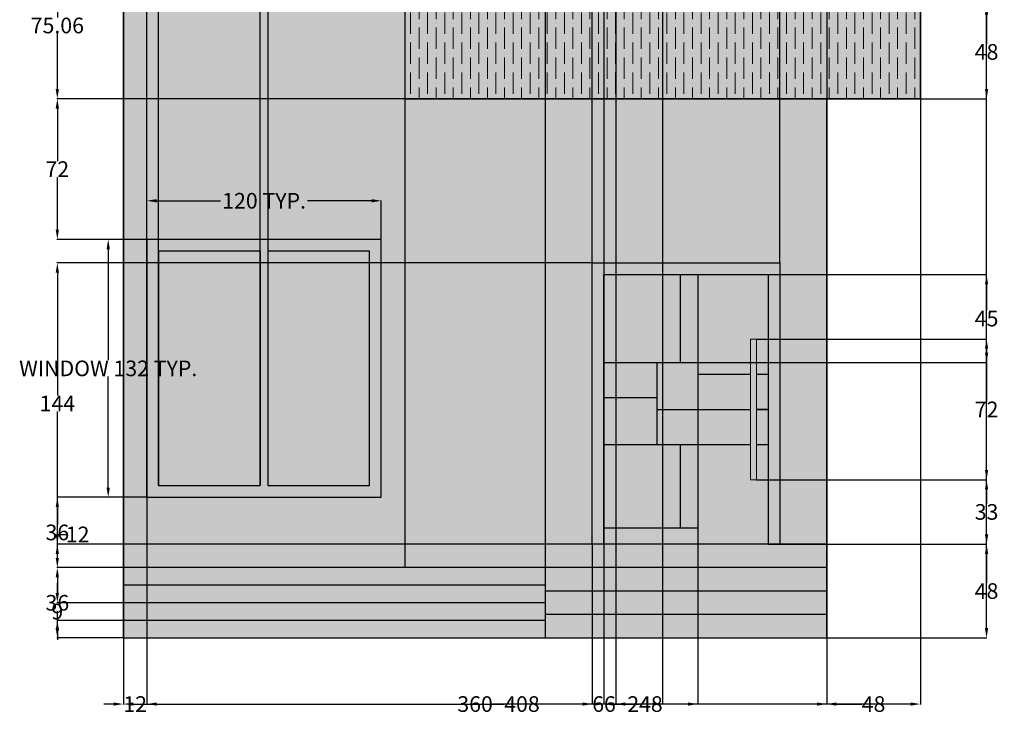
# Model space of a CAD drawing. Units: inches. Extents: x 137 to 641, y 88 to 838.
# Tile 1 of 2: x 137 to 641, y 88 to 444. Entities that reach past the tile are written whole.
import ezdxf

# ---------------------------------------------------------------- set-up
doc = ezdxf.new("R2010")
doc.units = ezdxf.units.IN
doc.header["$MEASUREMENT"] = 0
doc.layers.get('0').update_dxf_attribs({"color": 250})
for name, color, linetype, lineweight in [('A-ANNO-DIMS', 2, 'Continuous', 18), ('A-DOOR', 250, 'Continuous', 25), ('A-DOOR-HRDW', 250, 'Continuous', 18), ('A-ELEV-TRIM-PATT', 18, 'Continuous', 13), ('A-FLOR-BALC', 250, 'Continuous', 35), ('A-FLOR-BALC-PATT', 250, 'Continuous', 13), ('A-FLOR-STRS', 250, 'Continuous', 25), ('A-GLAZ', 250, 'Continuous', 25), ('A-GLAZ-PATT', 250, 'Continuous', 13), ('A-WALL', 250, 'Continuous', 35), ('A-WALL-CLAD', 250, 'Continuous', 25), ('A-WALL-PLIN', 251, 'Continuous', 25)]:
    doc.layers.add(name, color=color, linetype=linetype, lineweight=lineweight)
for name, color, linetype, lineweight, true_color in [('A-DOOR-PATT', 251, 'Continuous', 13, 0x636466), ('A-FLOR-BALC-FILL', 89, 'Continuous', 13, 0x333e19), ('A-FLOR-STRS-PATT', 9, 'Continuous', 13, 0xe0c8a3), ('A-WALL-CLAD-FILL', 51, 'Continuous', 13, 0xfff4a4), ('A-WALL-CLAD-PATT', 21, 'Continuous', 13, 0xe2a688), ('A-WALL-PATT', 254, 'Continuous', 13, 0xd7ebd2), ('A-WALL-PLIN-PATT', 108, 'Continuous', 13, 0x0a0f0b)]:
    doc.layers.add(name, color=color, linetype=linetype, lineweight=lineweight, true_color=true_color)
doc.styles.get("Standard").update_dxf_attribs({"font": 'arial.ttf'})
doc.dimstyles.get("Standard").update_dxf_attribs({"dimtxt": 8, "dimasz": 5, "dimexe": 0.18, "dimexo": 0.0625, "dimgap": 0.09, "dimtad": 0, "dimtih": 1, "dimtoh": 1, "dimdec": 0, "dimzin": 0, "dimdsep": 46, "dimlunit": 3, "dimtxsty": 'Standard', "dimcen": 0.09, "dimadec": 0, "dimazin": 0, "dimtfac": 1, "dimtdec": 0, "dimtofl": 0, "dimtmove": 0, "dimatfit": 3, "dimfxl": 1, "dimtolj": 1, "dimtzin": 0, "dimarcsym": 0})

# ---------------------------------------------------------------- blocks, each defined once
blk = doc.blocks.new('WIN-FRAME-2L-120X132')
for p, q in [((58, 126), (58, 6)), ((62, 126), (62, 6))]:
    blk.add_line(p, q)
for points in [[(120, 132), (0, 132)], [(0, 132), (0, 0), (120, 0), (120, 132)], [(58, 126), (6, 126)], [(6, 126), (6, 6), (58, 6)], [(62, 6), (114, 6), (114, 126)], [(114, 126), (62, 126)]]:
    blk.add_lwpolyline(points)
blk = doc.blocks.new('*D2')
at = {"layer": 'A-ANNO-DIMS', "color": 0, "lineweight": -2, "transparency": 16777216}
for p, q in [((201.86, 331.23), (181.95, 331.23)), ((182.13, 326.23), (182.13, 269.46)), ((182.13, 204.23), (182.13, 261)), ((201.86, 199.23), (181.95, 199.23))]:
    blk.add_line(p, q, dxfattribs=at)
at = {"layer": 'A-ANNO-DIMS', "color": 0, "transparency": 16777216}
for points in [[(181.29, 326.23), (182.96, 326.23), (182.13, 331.23)], [(181.29, 204.23), (182.96, 204.23), (182.13, 199.23)]]:
    blk.add_solid(points, dxfattribs=at)
at = {"layer": 'Defpoints', "color": 0, "transparency": 16777216}
for p in [(182.13, 331.23), (201.93, 331.23), (201.93, 199.23)]:
    blk.add_point(p, dxfattribs=at)
at = {"layer": 'A-ANNO-DIMS', "color": 0, "transparency": 16777216, "insert": (182.13, 265.23), "char_height": 8, "attachment_point": 5}
blk.add_mtext('\\A1;WINDOW 132 TYP.', dxfattribs=at)
blk = doc.blocks.new('*D3')
at = {"layer": 'A-ANNO-DIMS', "color": 0, "lineweight": -2, "transparency": 16777216}
for p, q in [((201.93, 331.29), (201.93, 351.21)), ((206.93, 351.03), (239.63, 351.03)), ((316.93, 351.03), (284.22, 351.03)), ((321.93, 331.29), (321.93, 351.21))]:
    blk.add_line(p, q, dxfattribs=at)
at = {"layer": 'A-ANNO-DIMS', "color": 0, "transparency": 16777216}
for points in [[(206.93, 351.86), (206.93, 350.2), (201.93, 351.03)], [(316.93, 351.86), (316.93, 350.2), (321.93, 351.03)]]:
    blk.add_solid(points, dxfattribs=at)
at = {"layer": 'Defpoints', "color": 0, "transparency": 16777216}
for p in [(321.93, 351.03), (201.93, 331.23), (321.93, 331.23)]:
    blk.add_point(p, dxfattribs=at)
at = {"layer": 'A-ANNO-DIMS', "color": 0, "transparency": 16777216, "insert": (261.93, 351.03), "char_height": 8, "attachment_point": 5}
blk.add_mtext('\\A1;120 TYP.', dxfattribs=at)
blk = doc.blocks.new('*D4')
at = {"layer": 'A-ANNO-DIMS', "color": 0, "lineweight": -2, "transparency": 16777216}
for p, q in [((597.93, 403.17), (597.93, 93.2)), ((189.93, 127.17), (189.93, 93.2)), ((194.93, 93.38), (384.83, 93.38)), ((592.93, 93.38), (403.02, 93.38))]:
    blk.add_line(p, q, dxfattribs=at)
at = {"layer": 'A-ANNO-DIMS', "color": 0, "transparency": 16777216}
for points in [[(194.93, 94.21), (194.93, 92.55), (189.93, 93.38)], [(592.93, 94.21), (592.93, 92.55), (597.93, 93.38)]]:
    blk.add_solid(points, dxfattribs=at)
at = {"layer": 'Defpoints', "color": 0, "transparency": 16777216}
for p in [(597.93, 403.23), (189.93, 127.23), (597.93, 93.38)]:
    blk.add_point(p, dxfattribs=at)
at = {"layer": 'A-ANNO-DIMS', "color": 0, "transparency": 16777216, "insert": (393.93, 93.38), "char_height": 8, "attachment_point": 5}
blk.add_mtext('\\A1;408', dxfattribs=at)
blk = doc.blocks.new('*D5')
at = {"layer": 'A-ANNO-DIMS', "color": 0, "lineweight": -2, "transparency": 16777216}
for p, q in [((333.99, 799.23), (631.96, 799.23)), ((631.78, 794.23), (631.78, 467.4)), ((631.78, 132.23), (631.78, 459.05)), ((549.99, 127.23), (631.96, 127.23))]:
    blk.add_line(p, q, dxfattribs=at)
at = {"layer": 'A-ANNO-DIMS', "color": 0, "transparency": 16777216}
for points in [[(630.94, 794.23), (632.61, 794.23), (631.78, 799.23)], [(630.94, 132.23), (632.61, 132.23), (631.78, 127.23)]]:
    blk.add_solid(points, dxfattribs=at)
at = {"layer": 'Defpoints', "color": 0, "transparency": 16777216}
for p in [(333.93, 799.23), (631.78, 799.23), (549.93, 127.23)]:
    blk.add_point(p, dxfattribs=at)
at = {"layer": 'A-ANNO-DIMS', "color": 0, "transparency": 16777216, "insert": (631.78, 463.23), "char_height": 8, "attachment_point": 5}
blk.add_mtext('\\A1;672', dxfattribs=at)
blk = doc.blocks.new('*D9')
at = {"layer": 'A-ANNO-DIMS', "color": 0, "lineweight": -2, "transparency": 16777216}
for p, q in [((333.86, 403.23), (155.9, 403.23)), ((156.08, 398.23), (156.08, 371.33)), ((156.08, 336.23), (156.08, 363.12)), ((201.86, 331.23), (155.9, 331.23))]:
    blk.add_line(p, q, dxfattribs=at)
at = {"layer": 'A-ANNO-DIMS', "color": 0, "transparency": 16777216}
for points in [[(155.24, 398.23), (156.91, 398.23), (156.08, 403.23)], [(155.24, 336.23), (156.91, 336.23), (156.08, 331.23)]]:
    blk.add_solid(points, dxfattribs=at)
at = {"layer": 'Defpoints', "color": 0, "transparency": 16777216}
for p in [(156.08, 403.23), (333.93, 403.23), (201.93, 331.23)]:
    blk.add_point(p, dxfattribs=at)
at = {"layer": 'A-ANNO-DIMS', "color": 0, "transparency": 16777216, "insert": (156.08, 367.23), "char_height": 8, "attachment_point": 5}
blk.add_mtext('\\A1;72', dxfattribs=at)
blk = doc.blocks.new('*D10')
at = {"layer": 'A-ANNO-DIMS', "color": 0, "lineweight": -2, "transparency": 16777216}
for p, q in [((201.86, 478.29), (155.9, 478.29)), ((156.08, 473.29), (156.08, 444.93)), ((156.08, 408.23), (156.08, 436.58)), ((333.86, 403.23), (155.9, 403.23))]:
    blk.add_line(p, q, dxfattribs=at)
at = {"layer": 'A-ANNO-DIMS', "color": 0, "transparency": 16777216}
for points in [[(155.24, 473.29), (156.91, 473.29), (156.08, 478.29)], [(155.24, 408.23), (156.91, 408.23), (156.08, 403.23)]]:
    blk.add_solid(points, dxfattribs=at)
at = {"layer": 'Defpoints', "color": 0, "transparency": 16777216}
for p in [(156.08, 478.29), (201.93, 478.29), (333.93, 403.23)]:
    blk.add_point(p, dxfattribs=at)
at = {"layer": 'A-ANNO-DIMS', "color": 0, "transparency": 16777216, "insert": (156.08, 440.76), "char_height": 8, "attachment_point": 5}
blk.add_mtext('\\A1;75.06', dxfattribs=at)
blk = doc.blocks.new('*D15')
at = {"layer": 'A-ANNO-DIMS', "color": 0, "lineweight": -2, "transparency": 16777216}
for p, q in [((189.93, 127.17), (189.93, 93.2)), ((549.93, 127.17), (549.93, 93.2)), ((194.93, 93.38), (361.01, 93.38)), ((544.93, 93.38), (378.84, 93.38))]:
    blk.add_line(p, q, dxfattribs=at)
at = {"layer": 'A-ANNO-DIMS', "color": 0, "transparency": 16777216}
for points in [[(194.93, 94.21), (194.93, 92.55), (189.93, 93.38)], [(544.93, 94.21), (544.93, 92.55), (549.93, 93.38)]]:
    blk.add_solid(points, dxfattribs=at)
at = {"layer": 'Defpoints', "color": 0, "transparency": 16777216}
for p in [(189.93, 127.23), (549.93, 127.23), (549.93, 93.38)]:
    blk.add_point(p, dxfattribs=at)
at = {"layer": 'A-ANNO-DIMS', "color": 0, "transparency": 16777216, "insert": (369.93, 93.38), "char_height": 8, "attachment_point": 5}
blk.add_mtext('\\A1;360', dxfattribs=at)
blk = doc.blocks.new('*D16')
at = {"layer": 'A-ANNO-DIMS', "color": 0, "lineweight": -2, "transparency": 16777216}
for p, q in [((201.93, 199.17), (201.93, 93.2)), ((189.93, 163.17), (189.93, 93.2)), ((184.93, 93.38), (179.93, 93.38)), ((206.93, 93.38), (211.93, 93.38))]:
    blk.add_line(p, q, dxfattribs=at)
at = {"layer": 'A-ANNO-DIMS', "color": 0, "transparency": 16777216}
for points in [[(184.93, 94.21), (184.93, 92.55), (189.93, 93.38)], [(206.93, 94.21), (206.93, 92.55), (201.93, 93.38)]]:
    blk.add_solid(points, dxfattribs=at)
at = {"layer": 'Defpoints', "color": 0, "transparency": 16777216}
for p in [(201.93, 199.23), (189.93, 163.23), (201.93, 93.38)]:
    blk.add_point(p, dxfattribs=at)
at = {"layer": 'A-ANNO-DIMS', "color": 0, "transparency": 16777216, "insert": (195.93, 93.38), "char_height": 8, "attachment_point": 5}
blk.add_mtext('\\A1;12', dxfattribs=at)
blk = doc.blocks.new('*D17')
at = {"layer": 'A-ANNO-DIMS', "color": 0, "lineweight": -2, "transparency": 16777216}
for p, q in [((201.86, 199.23), (155.9, 199.23)), ((156.08, 194.23), (156.08, 185.41)), ((156.08, 168.23), (156.08, 177.05)), ((189.86, 163.23), (155.9, 163.23))]:
    blk.add_line(p, q, dxfattribs=at)
at = {"layer": 'A-ANNO-DIMS', "color": 0, "transparency": 16777216}
for points in [[(155.24, 194.23), (156.91, 194.23), (156.08, 199.23)], [(155.24, 168.23), (156.91, 168.23), (156.08, 163.23)]]:
    blk.add_solid(points, dxfattribs=at)
at = {"layer": 'Defpoints', "color": 0, "transparency": 16777216}
for p in [(156.08, 199.23), (201.93, 199.23), (189.93, 163.23)]:
    blk.add_point(p, dxfattribs=at)
at = {"layer": 'A-ANNO-DIMS', "color": 0, "transparency": 16777216, "insert": (156.08, 181.23), "char_height": 8, "attachment_point": 5}
blk.add_mtext('\\A1;36', dxfattribs=at)
blk = doc.blocks.new('*D18')
at = {"layer": 'A-ANNO-DIMS', "color": 0, "lineweight": -2, "transparency": 16777216}
for p, q in [((189.86, 163.23), (155.9, 163.23)), ((156.08, 158.23), (156.08, 149.41)), ((156.08, 132.23), (156.08, 141.05)), ((189.86, 127.23), (155.9, 127.23))]:
    blk.add_line(p, q, dxfattribs=at)
at = {"layer": 'A-ANNO-DIMS', "color": 0, "transparency": 16777216}
for points in [[(155.24, 158.23), (156.91, 158.23), (156.08, 163.23)], [(155.24, 132.23), (156.91, 132.23), (156.08, 127.23)]]:
    blk.add_solid(points, dxfattribs=at)
at = {"layer": 'Defpoints', "color": 0, "transparency": 16777216}
for p in [(156.08, 163.23), (189.93, 163.23), (189.93, 127.23)]:
    blk.add_point(p, dxfattribs=at)
at = {"layer": 'A-ANNO-DIMS', "color": 0, "transparency": 16777216, "insert": (156.08, 145.23), "char_height": 8, "attachment_point": 5}
blk.add_mtext('\\A1;36', dxfattribs=at)
blk = doc.blocks.new('*D19')
at = {"layer": 'A-ANNO-DIMS', "color": 0, "lineweight": -2, "transparency": 16777216}
for p, q in [((156.08, 150.23), (156.08, 155.23)), ((405.86, 145.23), (155.9, 145.23)), ((405.86, 136.23), (155.9, 136.23)), ((156.08, 131.23), (156.08, 126.23))]:
    blk.add_line(p, q, dxfattribs=at)
at = {"layer": 'A-ANNO-DIMS', "color": 0, "transparency": 16777216}
for points in [[(155.24, 150.23), (156.91, 150.23), (156.08, 145.23)], [(155.24, 131.23), (156.91, 131.23), (156.08, 136.23)]]:
    blk.add_solid(points, dxfattribs=at)
at = {"layer": 'Defpoints', "color": 0, "transparency": 16777216}
for p in [(156.08, 145.23), (405.93, 145.23), (405.93, 136.23)]:
    blk.add_point(p, dxfattribs=at)
at = {"layer": 'A-ANNO-DIMS', "color": 0, "transparency": 16777216, "insert": (156.08, 140.73), "char_height": 8, "attachment_point": 5}
blk.add_mtext('\\A1;9', dxfattribs=at)
blk = doc.blocks.new('*D20')
at = {"layer": 'A-ANNO-DIMS', "color": 0, "lineweight": -2, "transparency": 16777216}
for p, q in [((405.93, 175.29), (405.93, 833.26)), ((410.93, 833.08), (412.05, 833.08)), ((424.93, 833.08), (423.8, 833.08)), ((429.93, 175.29), (429.93, 833.26))]:
    blk.add_line(p, q, dxfattribs=at)
at = {"layer": 'A-ANNO-DIMS', "color": 0, "transparency": 16777216}
for points in [[(410.93, 833.91), (410.93, 832.25), (405.93, 833.08)], [(424.93, 833.91), (424.93, 832.25), (429.93, 833.08)]]:
    blk.add_solid(points, dxfattribs=at)
at = {"layer": 'Defpoints', "color": 0, "transparency": 16777216}
for p in [(429.93, 833.08), (405.93, 175.23), (429.93, 175.23)]:
    blk.add_point(p, dxfattribs=at)
at = {"layer": 'A-ANNO-DIMS', "color": 0, "transparency": 16777216, "insert": (417.93, 833.08), "char_height": 8, "attachment_point": 5}
blk.add_mtext('\\A1;24', dxfattribs=at)
blk = doc.blocks.new('*D21')
at = {"layer": 'A-ANNO-DIMS', "color": 0, "lineweight": -2, "transparency": 16777216}
for p, q in [((429.93, 319.29), (429.93, 833.26)), ((434.93, 833.08), (472.11, 833.08)), ((520.93, 833.08), (483.74, 833.08)), ((525.93, 319.29), (525.93, 833.26))]:
    blk.add_line(p, q, dxfattribs=at)
at = {"layer": 'A-ANNO-DIMS', "color": 0, "transparency": 16777216}
for points in [[(434.93, 833.91), (434.93, 832.25), (429.93, 833.08)], [(520.93, 833.91), (520.93, 832.25), (525.93, 833.08)]]:
    blk.add_solid(points, dxfattribs=at)
at = {"layer": 'Defpoints', "color": 0, "transparency": 16777216}
for p in [(525.93, 833.08), (429.93, 319.23), (525.93, 319.23)]:
    blk.add_point(p, dxfattribs=at)
at = {"layer": 'A-ANNO-DIMS', "color": 0, "transparency": 16777216, "insert": (477.93, 833.08), "char_height": 8, "attachment_point": 5}
blk.add_mtext('\\A1;96', dxfattribs=at)
blk = doc.blocks.new('*D22')
at = {"layer": 'A-ANNO-DIMS', "color": 0, "lineweight": -2, "transparency": 16777216}
for p, q in [((429.86, 319.23), (155.9, 319.23)), ((156.08, 314.23), (156.08, 251.33)), ((156.08, 180.23), (156.08, 243.12)), ((429.86, 175.23), (155.9, 175.23))]:
    blk.add_line(p, q, dxfattribs=at)
at = {"layer": 'A-ANNO-DIMS', "color": 0, "transparency": 16777216}
for points in [[(155.24, 314.23), (156.91, 314.23), (156.08, 319.23)], [(155.24, 180.23), (156.91, 180.23), (156.08, 175.23)]]:
    blk.add_solid(points, dxfattribs=at)
at = {"layer": 'Defpoints', "color": 0, "transparency": 16777216}
for p in [(156.08, 319.23), (429.93, 319.23), (429.93, 175.23)]:
    blk.add_point(p, dxfattribs=at)
at = {"layer": 'A-ANNO-DIMS', "color": 0, "transparency": 16777216, "insert": (156.08, 247.23), "char_height": 8, "attachment_point": 5}
blk.add_mtext('\\A1;144', dxfattribs=at)
blk = doc.blocks.new('*D23')
at = {"layer": 'A-ANNO-DIMS', "color": 0, "lineweight": -2, "transparency": 16777216}
for p, q in [((549.99, 175.23), (631.96, 175.23)), ((631.78, 170.23), (631.78, 155.4)), ((631.78, 132.23), (631.78, 147.05)), ((549.99, 127.23), (631.96, 127.23))]:
    blk.add_line(p, q, dxfattribs=at)
at = {"layer": 'A-ANNO-DIMS', "color": 0, "transparency": 16777216}
for points in [[(630.94, 170.23), (632.61, 170.23), (631.78, 175.23)], [(630.94, 132.23), (632.61, 132.23), (631.78, 127.23)]]:
    blk.add_solid(points, dxfattribs=at)
at = {"layer": 'Defpoints', "color": 0, "transparency": 16777216}
for p in [(549.93, 175.23), (631.78, 175.23), (549.93, 127.23)]:
    blk.add_point(p, dxfattribs=at)
at = {"layer": 'A-ANNO-DIMS', "color": 0, "transparency": 16777216, "insert": (631.78, 151.23), "char_height": 8, "attachment_point": 5}
blk.add_mtext('\\A1;48', dxfattribs=at)
blk = doc.blocks.new('*D24')
at = {"layer": 'A-ANNO-DIMS', "color": 0, "lineweight": -2, "transparency": 16777216}
for p, q in [((156.08, 175.23), (156.08, 180.23)), ((156.08, 180.23), (161.08, 180.23)), ((549.86, 175.23), (155.9, 175.23)), ((156.08, 168.23), (156.08, 170.23)), ((549.86, 163.23), (155.9, 163.23))]:
    blk.add_line(p, q, dxfattribs=at)
at = {"layer": 'A-ANNO-DIMS', "color": 0, "transparency": 16777216}
for points in [[(155.24, 170.23), (156.91, 170.23), (156.08, 175.23)], [(155.24, 168.23), (156.91, 168.23), (156.08, 163.23)]]:
    blk.add_solid(points, dxfattribs=at)
at = {"layer": 'Defpoints', "color": 0, "transparency": 16777216}
for p in [(156.08, 175.23), (549.93, 175.23), (549.93, 163.23)]:
    blk.add_point(p, dxfattribs=at)
at = {"layer": 'A-ANNO-DIMS', "color": 0, "transparency": 16777216, "insert": (166.48, 180.23), "char_height": 8, "attachment_point": 5}
blk.add_mtext('\\A1;12', dxfattribs=at)
blk = doc.blocks.new('*D25')
at = {"layer": 'A-ANNO-DIMS', "color": 0, "lineweight": -2, "transparency": 16777216}
for p, q in [((429.93, 175.17), (429.93, 93.2)), ((435.93, 175.17), (435.93, 93.2)), ((424.93, 93.38), (419.93, 93.38)), ((440.93, 93.38), (445.93, 93.38))]:
    blk.add_line(p, q, dxfattribs=at)
at = {"layer": 'A-ANNO-DIMS', "color": 0, "transparency": 16777216}
for points in [[(424.93, 94.21), (424.93, 92.55), (429.93, 93.38)], [(440.93, 94.21), (440.93, 92.55), (435.93, 93.38)]]:
    blk.add_solid(points, dxfattribs=at)
at = {"layer": 'Defpoints', "color": 0, "transparency": 16777216}
for p in [(429.93, 175.23), (435.93, 175.23), (435.93, 93.38)]:
    blk.add_point(p, dxfattribs=at)
at = {"layer": 'A-ANNO-DIMS', "color": 0, "transparency": 16777216, "insert": (432.93, 93.38), "char_height": 8, "attachment_point": 5}
blk.add_mtext('\\A1;6', dxfattribs=at)
blk = doc.blocks.new('*D26')
at = {"layer": 'A-ANNO-DIMS', "color": 0, "lineweight": -2, "transparency": 16777216}
for p, q in [((435.93, 313.17), (435.93, 93.2)), ((483.93, 313.17), (483.93, 93.2)), ((440.93, 93.38), (453.94, 93.38)), ((478.93, 93.38), (465.91, 93.38))]:
    blk.add_line(p, q, dxfattribs=at)
at = {"layer": 'A-ANNO-DIMS', "color": 0, "transparency": 16777216}
for points in [[(440.93, 94.21), (440.93, 92.55), (435.93, 93.38)], [(478.93, 94.21), (478.93, 92.55), (483.93, 93.38)]]:
    blk.add_solid(points, dxfattribs=at)
at = {"layer": 'Defpoints', "color": 0, "transparency": 16777216}
for p in [(435.93, 313.23), (483.93, 313.23), (483.93, 93.38)]:
    blk.add_point(p, dxfattribs=at)
at = {"layer": 'A-ANNO-DIMS', "color": 0, "transparency": 16777216, "insert": (459.93, 93.38), "char_height": 8, "attachment_point": 5}
blk.add_mtext('\\A1;48', dxfattribs=at)
blk = doc.blocks.new('*D27')
at = {"layer": 'A-ANNO-DIMS', "color": 0, "lineweight": -2, "transparency": 16777216}
for p, q in [((435.99, 313.23), (631.96, 313.23)), ((631.78, 308.23), (631.78, 294.89)), ((631.78, 273.23), (631.78, 286.57)), ((435.99, 268.23), (631.96, 268.23))]:
    blk.add_line(p, q, dxfattribs=at)
at = {"layer": 'A-ANNO-DIMS', "color": 0, "transparency": 16777216}
for points in [[(630.94, 308.23), (632.61, 308.23), (631.78, 313.23)], [(630.94, 273.23), (632.61, 273.23), (631.78, 268.23)]]:
    blk.add_solid(points, dxfattribs=at)
at = {"layer": 'Defpoints', "color": 0, "transparency": 16777216}
for p in [(435.93, 313.23), (631.78, 313.23), (435.93, 268.23)]:
    blk.add_point(p, dxfattribs=at)
at = {"layer": 'A-ANNO-DIMS', "color": 0, "transparency": 16777216, "insert": (631.78, 290.73), "char_height": 8, "attachment_point": 5}
blk.add_mtext('\\A1;45', dxfattribs=at)
blk = doc.blocks.new('*D28')
at = {"layer": 'A-ANNO-DIMS', "color": 0, "lineweight": -2, "transparency": 16777216}
for p, q in [((513.99, 280.23), (631.96, 280.23)), ((631.78, 275.23), (631.78, 248.33)), ((631.78, 213.23), (631.78, 240.12)), ((513.99, 208.23), (631.96, 208.23))]:
    blk.add_line(p, q, dxfattribs=at)
at = {"layer": 'A-ANNO-DIMS', "color": 0, "transparency": 16777216}
for points in [[(630.94, 275.23), (632.61, 275.23), (631.78, 280.23)], [(630.94, 213.23), (632.61, 213.23), (631.78, 208.23)]]:
    blk.add_solid(points, dxfattribs=at)
at = {"layer": 'Defpoints', "color": 0, "transparency": 16777216}
for p in [(513.93, 280.23), (631.78, 280.23), (513.93, 208.23)]:
    blk.add_point(p, dxfattribs=at)
at = {"layer": 'A-ANNO-DIMS', "color": 0, "transparency": 16777216, "insert": (631.78, 244.23), "char_height": 8, "attachment_point": 5}
blk.add_mtext('\\A1;72', dxfattribs=at)
blk = doc.blocks.new('*D29')
at = {"layer": 'A-ANNO-DIMS', "color": 0, "lineweight": -2, "transparency": 16777216}
for p, q in [((513.99, 208.23), (631.96, 208.23)), ((631.78, 203.23), (631.78, 195.91)), ((631.78, 180.23), (631.78, 187.55)), ((519.99, 175.23), (631.96, 175.23))]:
    blk.add_line(p, q, dxfattribs=at)
at = {"layer": 'A-ANNO-DIMS', "color": 0, "transparency": 16777216}
for points in [[(630.94, 203.23), (632.61, 203.23), (631.78, 208.23)], [(630.94, 180.23), (632.61, 180.23), (631.78, 175.23)]]:
    blk.add_solid(points, dxfattribs=at)
at = {"layer": 'Defpoints', "color": 0, "transparency": 16777216}
for p in [(513.93, 208.23), (631.78, 208.23), (519.93, 175.23)]:
    blk.add_point(p, dxfattribs=at)
at = {"layer": 'A-ANNO-DIMS', "color": 0, "transparency": 16777216, "insert": (631.78, 191.73), "char_height": 8, "attachment_point": 5}
blk.add_mtext('\\A1;33', dxfattribs=at)
blk = doc.blocks.new('*D30')
at = {"layer": 'A-ANNO-DIMS', "color": 0, "lineweight": -2, "transparency": 16777216}
for p, q in [((196.93, 833.08), (191.93, 833.08)), ((201.93, 199.29), (201.93, 833.26)), ((207.93, 205.29), (207.93, 833.26)), ((212.93, 833.08), (217.93, 833.08))]:
    blk.add_line(p, q, dxfattribs=at)
at = {"layer": 'A-ANNO-DIMS', "color": 0, "transparency": 16777216}
for points in [[(196.93, 833.91), (196.93, 832.25), (201.93, 833.08)], [(212.93, 833.91), (212.93, 832.25), (207.93, 833.08)]]:
    blk.add_solid(points, dxfattribs=at)
at = {"layer": 'Defpoints', "color": 0, "transparency": 16777216}
for p in [(207.93, 833.08), (207.93, 205.23), (201.93, 199.23)]:
    blk.add_point(p, dxfattribs=at)
at = {"layer": 'A-ANNO-DIMS', "color": 0, "transparency": 16777216, "insert": (204.93, 833.08), "char_height": 8, "attachment_point": 5}
blk.add_mtext('\\A1;6', dxfattribs=at)
blk = doc.blocks.new('*D31')
at = {"layer": 'A-ANNO-DIMS', "color": 0, "lineweight": -2, "transparency": 16777216}
for p, q in [((254.93, 833.08), (249.93, 833.08)), ((259.93, 205.29), (259.93, 833.26)), ((263.93, 205.29), (263.93, 833.26)), ((268.93, 833.08), (273.93, 833.08))]:
    blk.add_line(p, q, dxfattribs=at)
at = {"layer": 'A-ANNO-DIMS', "color": 0, "transparency": 16777216}
for points in [[(254.93, 833.91), (254.93, 832.25), (259.93, 833.08)], [(268.93, 833.91), (268.93, 832.25), (263.93, 833.08)]]:
    blk.add_solid(points, dxfattribs=at)
at = {"layer": 'Defpoints', "color": 0, "transparency": 16777216}
for p in [(263.93, 833.08), (259.93, 205.23), (263.93, 205.23)]:
    blk.add_point(p, dxfattribs=at)
at = {"layer": 'A-ANNO-DIMS', "color": 0, "transparency": 16777216, "insert": (276.78, 833.08), "char_height": 8, "attachment_point": 5}
blk.add_mtext('\\A1;4', dxfattribs=at)
blk = doc.blocks.new('*D32')
at = {"layer": 'A-ANNO-DIMS', "color": 0, "lineweight": -2, "transparency": 16777216}
for p, q in [((549.93, 451.17), (549.93, 93.2)), ((597.93, 451.17), (597.93, 93.2)), ((554.93, 93.38), (567.94, 93.38)), ((592.93, 93.38), (579.91, 93.38))]:
    blk.add_line(p, q, dxfattribs=at)
at = {"layer": 'A-ANNO-DIMS', "color": 0, "transparency": 16777216}
for points in [[(554.93, 94.21), (554.93, 92.55), (549.93, 93.38)], [(592.93, 94.21), (592.93, 92.55), (597.93, 93.38)]]:
    blk.add_solid(points, dxfattribs=at)
at = {"layer": 'Defpoints', "color": 0, "transparency": 16777216}
for p in [(549.93, 451.23), (597.93, 451.23), (597.93, 93.38)]:
    blk.add_point(p, dxfattribs=at)
at = {"layer": 'A-ANNO-DIMS', "color": 0, "transparency": 16777216, "insert": (573.93, 93.38), "char_height": 8, "attachment_point": 5}
blk.add_mtext('\\A1;48', dxfattribs=at)
blk = doc.blocks.new('*D33')
at = {"layer": 'A-ANNO-DIMS', "color": 0, "lineweight": -2, "transparency": 16777216}
for p, q in [((597.99, 451.23), (631.96, 451.23)), ((631.78, 446.23), (631.78, 431.4)), ((631.78, 408.23), (631.78, 423.05)), ((597.99, 403.23), (631.96, 403.23))]:
    blk.add_line(p, q, dxfattribs=at)
at = {"layer": 'A-ANNO-DIMS', "color": 0, "transparency": 16777216}
for points in [[(630.94, 446.23), (632.61, 446.23), (631.78, 451.23)], [(630.94, 408.23), (632.61, 408.23), (631.78, 403.23)]]:
    blk.add_solid(points, dxfattribs=at)
at = {"layer": 'Defpoints', "color": 0, "transparency": 16777216}
for p in [(597.93, 451.23), (631.78, 451.23), (597.93, 403.23)]:
    blk.add_point(p, dxfattribs=at)
at = {"layer": 'A-ANNO-DIMS', "color": 0, "transparency": 16777216, "insert": (631.78, 427.23), "char_height": 8, "attachment_point": 5}
blk.add_mtext('\\A1;48', dxfattribs=at)
blk = doc.blocks.new('*D38')
at = {"layer": 'A-ANNO-DIMS', "color": 0, "lineweight": -2, "transparency": 16777216}
for p, q in [((435.93, 595.17), (435.93, 93.2)), ((441.93, 589.17), (441.93, 93.2)), ((430.93, 93.38), (425.93, 93.38)), ((446.93, 93.38), (451.93, 93.38))]:
    blk.add_line(p, q, dxfattribs=at)
at = {"layer": 'A-ANNO-DIMS', "color": 0, "transparency": 16777216}
for points in [[(430.93, 94.21), (430.93, 92.55), (435.93, 93.38)], [(446.93, 94.21), (446.93, 92.55), (441.93, 93.38)]]:
    blk.add_solid(points, dxfattribs=at)
at = {"layer": 'Defpoints', "color": 0, "transparency": 16777216}
for p in [(435.93, 595.23), (441.93, 589.23), (441.93, 93.38)]:
    blk.add_point(p, dxfattribs=at)
at = {"layer": 'A-ANNO-DIMS', "color": 0, "transparency": 16777216, "insert": (438.93, 93.38), "char_height": 8, "attachment_point": 5}
blk.add_mtext('\\A1;6', dxfattribs=at)
blk = doc.blocks.new('*D39')
at = {"layer": 'A-ANNO-DIMS', "color": 0, "lineweight": -2, "transparency": 16777216}
for p, q in [((441.93, 589.17), (441.93, 93.2)), ((465.93, 589.17), (465.93, 93.2)), ((446.93, 93.38), (448.05, 93.38)), ((460.93, 93.38), (459.8, 93.38))]:
    blk.add_line(p, q, dxfattribs=at)
at = {"layer": 'A-ANNO-DIMS', "color": 0, "transparency": 16777216}
for points in [[(446.93, 94.21), (446.93, 92.55), (441.93, 93.38)], [(460.93, 94.21), (460.93, 92.55), (465.93, 93.38)]]:
    blk.add_solid(points, dxfattribs=at)
at = {"layer": 'Defpoints', "color": 0, "transparency": 16777216}
for p in [(441.93, 589.23), (465.93, 589.23), (465.93, 93.38)]:
    blk.add_point(p, dxfattribs=at)
at = {"layer": 'A-ANNO-DIMS', "color": 0, "transparency": 16777216, "insert": (453.93, 93.38), "char_height": 8, "attachment_point": 5}
blk.add_mtext('\\A1;24', dxfattribs=at)

msp = doc.modelspace()

# ---------------------------------------------------------------- hatches: boundary and pattern name
at = {"layer": 'A-DOOR-PATT'}
h = msp.add_hatch(color=256, dxfattribs=at)
h.dxf.hatch_style = 1
h.paths.add_polyline_path([(474.925, 313.229), (435.925, 313.229), (435.925, 268.229), (474.925, 268.229)])
h.paths.add_polyline_path([(483.925, 313.229), (474.925, 313.229), (474.925, 268.229), (483.925, 268.229)])
h.paths.add_polyline_path([(519.925, 313.229), (483.925, 313.229), (483.925, 268.229), (483.925, 262.229), (510.925, 262.229), (510.925, 280.229), (513.925, 280.229), (513.925, 262.229), (519.925, 262.229)])
h.paths.add_polyline_path([(510.925, 262.229), (483.925, 262.229), (483.925, 244.229), (510.925, 244.229)])
h.paths.add_polyline_path([(483.925, 262.229), (483.925, 268.229), (474.925, 268.229), (462.925, 268.229), (462.925, 244.229), (483.925, 244.229)])
h.paths.add_polyline_path([(462.925, 268.229), (435.925, 268.229), (435.925, 250.229), (462.925, 250.229)])
h.paths.add_polyline_path([(462.925, 250.229), (435.925, 250.229), (435.925, 226.229), (462.925, 226.229)])
h.paths.add_polyline_path([(510.925, 244.229), (462.925, 244.229), (462.925, 226.229), (510.925, 226.229)])
h.paths.add_polyline_path([(474.925, 226.229), (462.925, 226.229), (435.925, 226.229), (435.925, 183.366), (474.925, 183.366)])
h.paths.add_polyline_path([(483.925, 183.366), (435.925, 183.366), (435.925, 175.229), (483.925, 175.229)])
h.paths.add_polyline_path([(483.925, 226.229), (474.925, 226.229), (474.925, 183.366), (483.925, 183.366)])
h.paths.add_polyline_path([(519.925, 226.229), (513.925, 226.229), (513.925, 208.229), (510.925, 208.229), (510.925, 226.229), (483.925, 226.229), (483.925, 183.366), (483.925, 175.229), (519.925, 175.229)])
h.paths.add_polyline_path([(519.925, 244.229), (513.925, 244.229), (513.925, 226.229), (519.925, 226.229)])
h.paths.add_polyline_path([(519.925, 262.229), (513.925, 262.229), (513.925, 244.229), (519.925, 244.229)])
at = {"layer": 'A-ELEV-TRIM-PATT'}
h = msp.add_hatch(color=256, dxfattribs=at)
h.dxf.hatch_style = 1
h.paths.add_polyline_path([(321.925, 610.288), (201.925, 610.288), (201.925, 478.288), (321.925, 478.288)])
h.paths.add_polyline_path([(263.925, 484.288), (263.925, 604.288), (315.925, 604.288), (315.925, 484.288)], flags=16)
h.paths.add_polyline_path([(259.925, 484.288), (207.925, 484.288), (207.925, 604.288), (259.925, 604.288)], flags=16)
h.paths.add_polyline_path([(321.925, 331.229), (201.925, 331.229), (201.925, 199.229), (321.925, 199.229)])
h.paths.add_polyline_path([(263.925, 325.229), (315.925, 325.229), (315.925, 205.229), (263.925, 205.229)], flags=16)
h.paths.add_polyline_path([(259.925, 325.229), (259.925, 205.229), (207.925, 205.229), (207.925, 325.229)], flags=16)
h = msp.add_hatch(color=256, dxfattribs=at)
h.dxf.hatch_style = 1
h.paths.add_polyline_path([(525.925, 319.229), (429.925, 319.229), (429.925, 175.229), (435.925, 175.229), (435.925, 313.229), (519.925, 313.229), (519.925, 175.229), (525.925, 175.229)])
h.paths.add_polyline_path([(513.925, 280.229), (510.925, 280.229), (510.925, 208.229), (513.925, 208.229), (513.925, 244.229)], flags=17)
h.paths.add_polyline_path([(519.925, 595.229), (435.925, 595.229), (435.925, 505.229), (441.925, 505.229), (441.925, 589.229), (513.925, 589.229), (513.925, 505.229), (519.925, 505.229)])
h.paths.add_polyline_path([(519.925, 505.229), (513.925, 505.229), (513.925, 454.229), (441.925, 454.229), (441.925, 505.229), (435.925, 505.229), (435.925, 451.229), (519.925, 451.229)])
at = {"layer": 'A-FLOR-BALC-FILL'}
msp.add_hatch(color=256, dxfattribs=at).paths.add_polyline_path([(597.925, 451.229), (549.925, 451.229), (333.925, 451.229), (333.925, 403.229), (549.925, 403.229), (597.925, 403.229)])
at = {"layer": 'A-FLOR-BALC-PATT'}
h = msp.add_hatch(dxfattribs=at)
h.set_pattern_fill('ANSI36', color=256, scale=35, angle=45, style=0)
h.paths.add_polyline_path([(597.925, 451.229), (549.925, 451.229), (333.925, 451.229), (333.925, 403.229), (549.925, 403.229), (597.925, 403.229)])
at = {"layer": 'A-FLOR-STRS-PATT'}
msp.add_hatch(color=256, dxfattribs=at).paths.add_polyline_path([(549.925, 175.229), (405.925, 175.229), (405.925, 163.229), (549.925, 163.229)])
h = msp.add_hatch(color=256, dxfattribs=at)
h.paths.add_polyline_path([(549.925, 163.229), (405.925, 163.229), (405.925, 151.229), (549.925, 151.229)])
h.paths.add_polyline_path([(549.925, 151.229), (405.925, 151.229), (405.925, 139.229), (549.925, 139.229)])
h.paths.add_polyline_path([(549.925, 139.229), (405.925, 139.229), (405.925, 127.229), (549.925, 127.229)])
at = {"layer": 'A-GLAZ-PATT'}
h = msp.add_hatch(color=256, dxfattribs=at)
h.set_gradient(color1=(199, 200, 202), color2=(147, 149, 152), rotation=45, name='INVCYLINDER')
h.paths.add_polyline_path([(315.925, 325.229), (263.925, 325.229), (263.925, 205.229), (315.925, 205.229)])
h.paths.add_polyline_path([(259.925, 325.229), (207.925, 325.229), (207.925, 205.229), (259.925, 205.229)])
at = {"layer": 'A-WALL-CLAD-FILL'}
h = msp.add_hatch(color=256, dxfattribs=at)
h.paths.add_polyline_path([(405.925, 691.229), (333.925, 691.229), (333.925, 505.229), (405.925, 505.229)])
h.paths.add_polyline_path([(405.925, 505.229), (333.925, 505.229), (333.925, 451.229), (405.925, 451.229)])
h.paths.add_polyline_path([(405.925, 403.229), (333.925, 403.229), (333.925, 163.229), (405.925, 163.229)])
at = {"layer": 'A-WALL-CLAD-PATT'}
h = msp.add_hatch(dxfattribs=at)
h.set_pattern_fill('GRAVEL', color=256, scale=15, style=0)
h.set_pattern_definition([(228.01279, (10.8, 15), (-120, -135), [2.01804, -199.78632]), (184.96974, (9.45, 13.5), (180, 15), [3.46302, -342.83887]), (132.51045, (6, 13.2), (150, -165), [2.44182, -241.74049]), (267.27369, (0.15, 9.45), (15, 300), [3.15357, -312.20337]), (292.83365, (0, 6.3), (-75, 180), [3.09232, -306.1406]), (357.27369, (1.2, 3.45), (-300, 15), [3.15357, -312.20337]), (37.69424, (4.35, 3.3), (-195, -150), [4.17043, -412.87273]), (72.25533, (7.65, 5.85), (105, 330), [3.93732, -389.79482]), (121.42957, (8.85, 9.6), (-120, 195), [3.16425, -313.2611]), (175.23636, (7.2, 12.3), (165, -15), [3.61248, -177.01144]), (222.39744, (3.6, 12.6), (-180, -165), [4.67172, -462.50063]), (138.81407, (15, 9.3), (-105, 90), [1.59451, -157.85767]), (171.46923, (13.8, 10.35), (195, -30), [3.03355, -300.32267]), (225, (10.8, 10.8), (-2e-15, -15), [2.12132, -19.0919]), (203.1986, (9.75, 12.6), (75, 30), [1.14237, -113.09423]), (291.8014, (8.7, 12.15), (-15, 45), [1.61555, -79.16193]), (30.96376, (9.3, 10.65), (45, 30), [2.62393, -84.84034]), (161.56505, (11.55, 12), (30, -15), [1.89736, -45.5368]), (16.38954, (0, 12.15), (150, 45), [2.658, -263.14268]), (70.34618, (2.55, 12.9), (-60, -165), [2.22991, -220.76112]), (293.1986, (11.55, 15), (-30, 75), [2.28472, -111.95187]), (343.61046, (12.45, 12.9), (-150, 45), [2.658, -263.14268]), (339.44395, (0, 2.85), (-75, 30), [2.5632, -125.59686]), (294.77514, (2.4, 1.95), (-75, 165), [2.14767, -212.61965]), (66.8014, (11.7, 0), (30, 75), [2.28472, -111.95187]), (17.35402, (12.6, 2.1), (-195, -60), [2.51446, -248.93135]), (69.44395, (4.35, 0), (-30, -75), [1.2816, -126.87846]), (101.30993, (10.8, 0), (-15, 60), [0.76485, -75.72044]), (165.96376, (10.65, 0.75), (45, -15), [3.09233, -58.75426]), (186.00901, (7.65, 1.5), (150, 15), [2.86575, -283.70885]), (303.69007, (9.3, 9.3), (-15, 30), [2.16333, -51.91994]), (353.15723, (10.5, 7.5), (255, -30), [3.77691, -373.91344]), (60.9454, (14.25, 7.05), (-60, -105), [1.54434, -152.89011]), (90, (15, 8.4), (-15, 15), [0.9, -14.1]), (120.25644, (7.35, 1.95), (60, -105), [2.08386, -206.3028]), (48.01279, (6.3, 3.75), (120, 135), [4.03608, -197.76828]), (0, (9, 6.75), (15, 15), [3.9, -11.1]), (325.30485, (12.9, 6.75), (150, -105), [2.3717, -234.79911]), (254.0546, (14.85, 5.4), (-15, -60), [2.18403, -107.01762]), (207.645975, (14.25, 3.3), (-285, -150), [3.55598, -352.04211]), (175.42608, (11.1, 1.65), (-195, 15), [3.76199, -372.4361])])
h.paths.add_polyline_path([(405.925, 691.229), (333.925, 691.229), (333.925, 505.229), (405.925, 505.229)])
h.paths.add_polyline_path([(405.925, 505.229), (333.925, 505.229), (333.925, 451.229), (405.925, 451.229)])
h.paths.add_polyline_path([(405.925, 403.229), (333.925, 403.229), (333.925, 163.229), (405.925, 163.229)])
at = {"layer": 'A-WALL-PATT'}
h = msp.add_hatch(color=256, dxfattribs=at)
h.dxf.hatch_style = 1
h.paths.add_polyline_path([(189.925, 163.229), (333.925, 163.229), (333.925, 691.229), (189.925, 691.229)])
h.paths.add_polyline_path([(201.925, 478.288), (201.925, 610.288), (321.925, 610.288), (321.925, 478.288)], flags=16)
h.paths.add_polyline_path([(207.925, 484.288), (207.925, 604.288), (259.925, 604.288), (259.925, 484.288)], flags=0)
h.paths.add_polyline_path([(263.925, 484.288), (263.925, 604.288), (315.925, 604.288), (315.925, 484.288)], flags=0)
h.paths.add_polyline_path([(321.925, 331.229), (321.925, 199.229), (201.925, 199.229), (201.925, 331.229)], flags=16)
h.paths.add_polyline_path([(259.925, 325.229), (259.925, 205.229), (207.925, 205.229), (207.925, 325.229)], flags=0)
h.paths.add_polyline_path([(263.925, 325.229), (315.925, 325.229), (315.925, 205.229), (263.925, 205.229)], flags=0)
h = msp.add_hatch(color=256, dxfattribs=at)
h.set_gradient(color1=(199, 200, 202), color2=(147, 149, 152), name='INVCYLINDER')
h.paths.add_polyline_path([(405.925, 403.229), (405.925, 175.229), (429.925, 175.229), (429.925, 319.229), (525.925, 319.229), (525.925, 175.229), (549.925, 175.229), (549.925, 403.229)])
at = {"layer": 'A-WALL-PLIN-PATT'}
h = msp.add_hatch(color=256, dxfattribs=at)
h.paths.add_polyline_path([(405.925, 163.229), (189.925, 163.229), (189.925, 154.229), (405.925, 154.229)])
h.paths.add_polyline_path([(405.925, 154.229), (189.925, 154.229), (189.925, 145.229), (405.925, 145.229)])
h.paths.add_polyline_path([(405.925, 145.229), (189.925, 145.229), (189.925, 136.229), (405.925, 136.229)])
h.paths.add_polyline_path([(405.925, 136.229), (189.925, 136.229), (189.925, 127.229), (405.925, 127.229)])

# ---------------------------------------------------------------- linework, layer by layer
at = {"layer": 'A-DOOR'}
for p, q in [((429.925, 319.229), (525.925, 319.229)), ((429.925, 175.229), (429.925, 319.229)), ((525.925, 319.229), (525.925, 175.229)), ((435.925, 175.229), (435.925, 313.229)), ((435.925, 313.229), (519.925, 313.229)), ((474.925, 313.229), (474.925, 268.229)), ((483.925, 313.229), (483.925, 244.229)), ((519.925, 313.229), (519.925, 175.229)), ((435.925, 268.229), (483.925, 268.229)), ((462.925, 268.229), (462.925, 226.229)), ((483.925, 262.229), (510.925, 262.229)), ((513.925, 262.229), (519.925, 262.229)), ((435.925, 250.229), (462.925, 250.229)), ((462.925, 244.229), (510.925, 244.229)), ((519.925, 244.229), (513.925, 244.229)), ((513.925, 244.229), (519.925, 244.229)), ((435.925, 226.229), (510.925, 226.229)), ((474.925, 226.229), (474.925, 183.366)), ((483.925, 226.229), (483.925, 175.229)), ((513.925, 226.229), (519.925, 226.229)), ((483.925, 183.366), (435.925, 183.366))]:
    msp.add_line(p, q, dxfattribs=at)
at = {"layer": 'A-DOOR-HRDW'}
for p, q in [((513.925, 280.229), (510.925, 280.229)), ((510.925, 280.229), (510.925, 208.229)), ((513.925, 244.229), (513.925, 280.229)), ((513.925, 208.229), (513.925, 244.229)), ((510.925, 208.229), (513.925, 208.229))]:
    msp.add_line(p, q, dxfattribs=at)
at = {"layer": 'A-FLOR-BALC'}
for p, q in [((597.925, 451.229), (597.925, 403.229)), ((549.925, 403.229), (333.925, 403.229)), ((597.925, 403.229), (549.925, 403.229))]:
    msp.add_line(p, q, dxfattribs=at)
at = {"layer": 'A-FLOR-STRS'}
for p, q in [((549.925, 175.229), (405.925, 175.229)), ((549.925, 151.229), (405.925, 151.229)), ((549.925, 139.229), (405.925, 139.229))]:
    msp.add_line(p, q, dxfattribs=at)
at = {"layer": 'A-WALL'}
for p, q in [((189.925, 727.229), (189.925, 127.229)), ((549.925, 127.229), (549.925, 403.229))]:
    msp.add_line(p, q, dxfattribs=at)
at = {"layer": 'A-WALL-CLAD'}
for p, q in [((333.925, 691.229), (333.925, 163.229)), ((405.925, 127.229), (405.925, 403.229))]:
    msp.add_line(p, q, dxfattribs=at)
at = {"layer": 'A-WALL-PLIN'}
for p, q in [((549.925, 163.229), (189.925, 163.229)), ((405.925, 154.229), (189.925, 154.229)), ((405.925, 145.229), (189.925, 145.229)), ((405.925, 136.229), (189.925, 136.229)), ((189.925, 127.229), (549.925, 127.229))]:
    msp.add_line(p, q, dxfattribs=at)

# ---------------------------------------------------------------- block references
at = {"layer": 'A-GLAZ'}
msp.add_blockref('WIN-FRAME-2L-120X132', (201.925, 199.229), dxfattribs=at)

# ---------------------------------------------------------------- dimensions: what is measured, and where the dimension line sits
at = {"layer": 'A-ANNO-DIMS'}
for base, p1, p2, picture, middle in [((207.925, 833.079), (201.925, 199.229), (207.925, 205.229), '*D30', (204.925, 833.079)), ((263.925, 833.079), (259.925, 205.229), (263.925, 205.229), '*D31', (276.782, 833.079)), ((429.925, 833.079), (405.925, 175.229), (429.925, 175.229), '*D20', (417.925, 833.079)), ((525.925, 833.079), (429.925, 319.229), (525.925, 319.229), '*D21', (477.925, 833.079)), ((441.925, 93.379), (435.925, 595.229), (441.925, 589.229), '*D38', (438.925, 93.379)), ((465.925, 93.379), (441.925, 589.229), (465.925, 589.229), '*D39', (453.925, 93.379)), ((597.925, 93.379), (549.925, 451.229), (597.925, 451.229), '*D32', (573.925, 93.379)), ((597.925, 93.379), (189.925, 127.229), (597.925, 403.229), '*D4', (393.925, 93.379)), ((483.925, 93.379), (435.925, 313.229), (483.925, 313.229), '*D26', (459.925, 93.379)), ((201.925, 93.379), (189.925, 163.229), (201.925, 199.229), '*D16', (195.925, 93.379)), ((435.925, 93.379), (429.925, 175.229), (435.925, 175.229), '*D25', (432.925, 93.379)), ((549.925, 93.379), (189.925, 127.229), (549.925, 127.229), '*D15', (369.925, 93.379))]:
    dim = msp.add_linear_dim(base=base, p1=p1, p2=p2, dimstyle='Standard', override={"dimdec": 0, "dimlfac": 1, "dimrnd": 0, "dimzin": 0, "dimdsep": 46, "dimlunit": 2}, dxfattribs=at)
    dim.commit()
    dim.dimension.update_dxf_attribs({"geometry": picture, "text_midpoint": middle})
for base, p1, p2, override, picture, middle in [((631.775, 799.229), (549.925, 127.229), (333.925, 799.229), {"dimdec": 0, "dimlfac": 1, "dimrnd": 0, "dimzin": 0, "dimdsep": 46, "dimlunit": 2}, '*D5', (631.775, 463.229)), ((156.075, 478.288), (333.925, 403.229), (201.925, 478.288), {"dimdec": 2, "dimlfac": 1, "dimrnd": 0, "dimzin": 0, "dimdsep": 46, "dimlunit": 2}, '*D10', (156.075, 440.758)), ((631.775, 451.229), (597.925, 403.229), (597.925, 451.229), {"dimdec": 0, "dimlfac": 1, "dimrnd": 0, "dimzin": 0, "dimdsep": 46, "dimlunit": 2}, '*D33', (631.775, 427.229)), ((156.075, 403.229), (201.925, 331.229), (333.925, 403.229), {"dimdec": 0, "dimlfac": 1, "dimrnd": 0, "dimzin": 0, "dimdsep": 46, "dimlunit": 2}, '*D9', (156.075, 367.229)), ((156.075, 319.229), (429.925, 175.229), (429.925, 319.229), {"dimdec": 0, "dimlfac": 1, "dimrnd": 0, "dimzin": 0, "dimdsep": 46, "dimlunit": 2}, '*D22', (156.075, 247.229)), ((631.775, 313.229), (435.925, 268.229), (435.925, 313.229), {"dimdec": 0, "dimlfac": 1, "dimrnd": 0, "dimzin": 0, "dimdsep": 46, "dimlunit": 2}, '*D27', (631.775, 290.729)), ((631.775, 280.229), (513.925, 208.229), (513.925, 280.229), {"dimdec": 0, "dimlfac": 1, "dimrnd": 0, "dimzin": 0, "dimdsep": 46, "dimlunit": 2}, '*D28', (631.775, 244.229)), ((631.775, 208.229), (519.925, 175.229), (513.925, 208.229), {"dimdec": 0, "dimlfac": 1, "dimrnd": 0, "dimzin": 0, "dimdsep": 46, "dimlunit": 2}, '*D29', (631.775, 191.729)), ((156.075, 199.229), (189.925, 163.229), (201.925, 199.229), {"dimdec": 0, "dimlfac": 1, "dimrnd": 0, "dimzin": 0, "dimdsep": 46, "dimlunit": 2}, '*D17', (156.075, 181.229)), ((156.075, 175.229), (549.925, 163.229), (549.925, 175.229), {"dimdec": 0, "dimlfac": 1, "dimrnd": 0, "dimzin": 0, "dimdsep": 46, "dimlunit": 2}, '*D24', (166.478, 180.229)), ((631.775, 175.229), (549.925, 127.229), (549.925, 175.229), {"dimdec": 0, "dimlfac": 1, "dimrnd": 0, "dimzin": 0, "dimdsep": 46, "dimlunit": 2}, '*D23', (631.775, 151.229)), ((156.075, 163.229), (189.925, 127.229), (189.925, 163.229), {"dimdec": 0, "dimlfac": 1, "dimrnd": 0, "dimzin": 0, "dimdsep": 46, "dimlunit": 2}, '*D18', (156.075, 145.229)), ((156.075, 145.229), (405.925, 136.229), (405.925, 145.229), {"dimdec": 0, "dimlfac": 1, "dimrnd": 0, "dimzin": 0, "dimdsep": 46, "dimlunit": 2}, '*D19', (156.075, 140.729))]:
    dim = msp.add_linear_dim(base=base, p1=p1, p2=p2, angle=90, dimstyle='Standard', override=override, dxfattribs=at)
    dim.commit()
    dim.dimension.update_dxf_attribs({"geometry": picture, "text_midpoint": middle})
dim = msp.add_linear_dim(base=(321.925, 351.029), p1=(201.925, 331.229), p2=(321.925, 331.229), text='<> TYP.', dimstyle='Standard', override={"dimdec": 0, "dimlfac": 1, "dimrnd": 0, "dimzin": 0, "dimdsep": 46, "dimlunit": 2}, dxfattribs=at)
dim.commit()
dim.dimension.update_dxf_attribs({"geometry": '*D3', "text_midpoint": (261.925, 351.029)})
dim = msp.add_linear_dim(base=(182.125, 331.229), p1=(201.925, 199.229), p2=(201.925, 331.229), angle=90, text='WINDOW <> TYP.', dimstyle='Standard', override={"dimdec": 0, "dimlfac": 1, "dimrnd": 0, "dimzin": 0, "dimdsep": 46, "dimlunit": 2}, dxfattribs=at)
dim.commit()
dim.dimension.update_dxf_attribs({"geometry": '*D2', "text_midpoint": (182.125, 265.229)})

doc.saveas('drawing.dxf')
